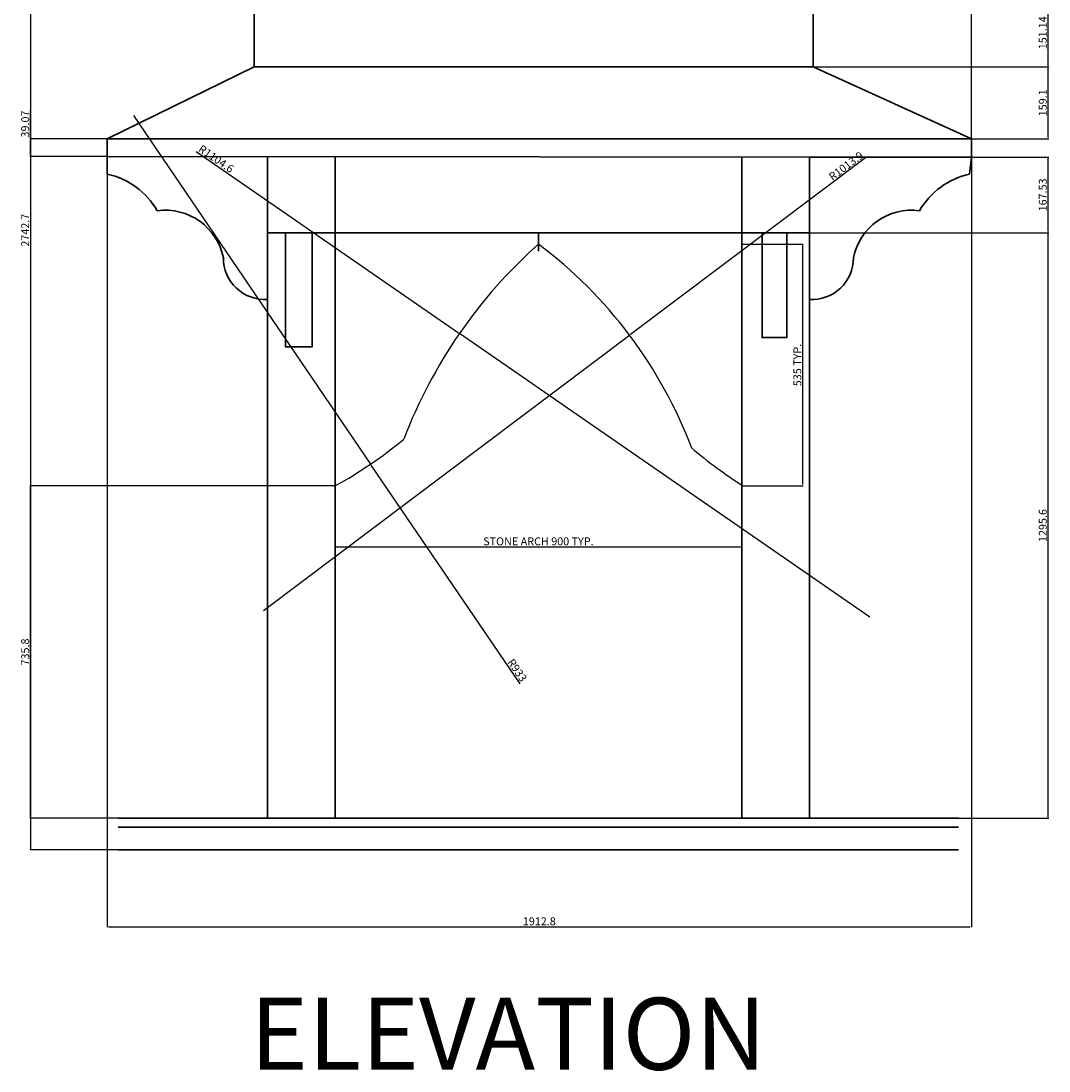
# Model space of a CAD drawing. Units: millimetres. Extents: x 498 to 8860, y -426 to 8717.
# Tile 8 of 9: x 4984 to 7260, y 3757 to 6081. Entities that reach past the tile are written whole.
import ezdxf

# ---------------------------------------------------------------- set-up
doc = ezdxf.new("R2010")
doc.units = ezdxf.units.MM
for name, color, linetype, lineweight in [('A-ANNO-DIMS', 2, 'Continuous', 18), ('A-ANNO-TEXT', 3, 'Continuous', 18), ('A-DETL', 7, 'Continuous', 25), ('A-ELEV', 7, 'Continuous', 35)]:
    doc.layers.add(name, color=color, linetype=linetype, lineweight=lineweight)
doc.styles.get("Standard").update_dxf_attribs({"font": 'arial.ttf'})
doc.dimstyles.new('ISO-25', dxfattribs={"dimtxt": 17.5, "dimasz": 2.5, "dimexe": 1.25, "dimexo": 0.625, "dimtad": 1, "dimdec": 0, "dimtxsty": 'Standard', "dimcen": 2.5, "dimadec": 0, "dimazin": 0, "dimtfac": 1, "dimtdec": 0, "dimtmove": 0, "dimatfit": 3, "dimfxl": 1, "dimarcsym": 0})

# ---------------------------------------------------------------- blocks, each defined once
blk = doc.blocks.new('BRACKET-STONE')
for centre, radius, start, end in [((1183.8, -291.1), 1104.6, 131.6209, 159.0769), ((-158.8, -276), 1013.9, 20.7397, 53.0882), ((-446.2, 819.4), 933, 298.5683, 309.875), ((1523.8, 965), 1147.7, 230.2129, 237.0762)]:
    blk.add_arc(centre, radius, start, end)
blk = doc.blocks.new('*D41')
at = {"layer": 'A-ANNO-DIMS', "color": 0, "lineweight": -2, "transparency": 16777216}
for p, q in [((5679.7, 5051.8), (5679.7, 4916.1)), ((6579.7, 5051.8), (6579.7, 4916.1)), ((5682.2, 4917.4), (6577.2, 4917.4))]:
    blk.add_line(p, q, dxfattribs=at)
at = {"layer": 'A-ANNO-DIMS', "color": 0, "transparency": 16777216}
for points in [[(5682.2, 4917.8), (5682.2, 4917), (5679.7, 4917.4)], [(6577.2, 4917.8), (6577.2, 4917), (6579.7, 4917.4)]]:
    blk.add_solid(points, dxfattribs=at)
at = {"layer": 'Defpoints', "color": 0, "transparency": 16777216}
for p in [(5679.7, 5052.4), (6579.7, 5052.4), (6579.7, 4917.4)]:
    blk.add_point(p, dxfattribs=at)
at = {"layer": 'A-ANNO-DIMS', "color": 0, "transparency": 16777216, "insert": (6129.7, 4927.1), "char_height": 17.5, "attachment_point": 5}
blk.add_mtext('STONE ARCH 900 TYP.', dxfattribs=at)
blk = doc.blocks.new('*D42')
at = {"layer": 'A-ANNO-DIMS', "color": 0, "lineweight": -2, "transparency": 16777216}
for p, q in [((6580.4, 5587.1), (6716, 5587.1)), ((6714.7, 5054.9), (6714.7, 5584.6)), ((6580.4, 5052.4), (6716, 5052.4))]:
    blk.add_line(p, q, dxfattribs=at)
at = {"layer": 'A-ANNO-DIMS', "color": 0, "transparency": 16777216}
for points in [[(6714.3, 5584.6), (6715.1, 5584.6), (6714.7, 5587.1)], [(6714.3, 5054.9), (6715.1, 5054.9), (6714.7, 5052.4)]]:
    blk.add_solid(points, dxfattribs=at)
at = {"layer": 'Defpoints', "color": 0, "transparency": 16777216}
for p in [(6579.7, 5587.1), (6714.7, 5587.1), (6579.7, 5052.4)]:
    blk.add_point(p, dxfattribs=at)
at = {"layer": 'A-ANNO-DIMS', "color": 0, "transparency": 16777216, "insert": (6705.2, 5319.7), "char_height": 17.5, "attachment_point": 5, "rotation": 90}
blk.add_mtext('535 TYP.', dxfattribs=at)
blk = doc.blocks.new('*D52')
at = {"layer": 'A-ANNO-DIMS', "color": 0, "lineweight": -2, "transparency": 16777216}
for p, q in [((5175.3, 5819.6), (5175.3, 4075.4)), ((7088.1, 5819.6), (7088.1, 4075.4)), ((5177.8, 4076.6), (7085.6, 4076.6))]:
    blk.add_line(p, q, dxfattribs=at)
at = {"layer": 'A-ANNO-DIMS', "color": 0, "transparency": 16777216}
for points in [[(5177.8, 4077), (5177.8, 4076.2), (5175.3, 4076.6)], [(7085.6, 4077), (7085.6, 4076.2), (7088.1, 4076.6)]]:
    blk.add_solid(points, dxfattribs=at)
at = {"layer": 'Defpoints', "color": 0, "transparency": 16777216}
for p in [(5175.3, 5820.3), (7088.1, 5820.3), (7088.1, 4076.6)]:
    blk.add_point(p, dxfattribs=at)
at = {"layer": 'A-ANNO-DIMS', "color": 0, "transparency": 16777216, "insert": (6131.7, 4086.2), "char_height": 17.5, "attachment_point": 5}
blk.add_mtext('1912.8', dxfattribs=at)
blk = doc.blocks.new('*D53')
at = {"layer": 'A-ANNO-DIMS', "color": 0, "lineweight": -2, "transparency": 16777216}
for p, q in [((6135.6, 6989.3), (5004.1, 6989.3)), ((5005.3, 6986.8), (5005.3, 4249.1)), ((5199.1, 4246.6), (5004.1, 4246.6))]:
    blk.add_line(p, q, dxfattribs=at)
at = {"layer": 'A-ANNO-DIMS', "color": 0, "transparency": 16777216}
for points in [[(5004.9, 6986.8), (5005.8, 6986.8), (5005.3, 6989.3)], [(5004.9, 4249.1), (5005.8, 4249.1), (5005.3, 4246.6)]]:
    blk.add_solid(points, dxfattribs=at)
at = {"layer": 'Defpoints', "color": 0, "transparency": 16777216}
for p in [(6136.2, 6989.3), (5005.3, 4246.6), (5199.7, 4246.6)]:
    blk.add_point(p, dxfattribs=at)
at = {"layer": 'A-ANNO-DIMS', "color": 0, "transparency": 16777216, "insert": (4995.9, 5617.9), "char_height": 17.5, "attachment_point": 5, "rotation": 90}
blk.add_mtext('2742.7', dxfattribs=at)
blk = doc.blocks.new('*D54')
at = {"layer": 'A-ANNO-DIMS', "color": 0, "lineweight": -2, "transparency": 16777216}
for p, q in [((6730.4, 5612.2), (7259.3, 5612.2)), ((7258.1, 4319.1), (7258.1, 5609.7)), ((6730.4, 4316.6), (7259.3, 4316.6))]:
    blk.add_line(p, q, dxfattribs=at)
at = {"layer": 'A-ANNO-DIMS', "color": 0, "transparency": 16777216}
for points in [[(7257.7, 5609.7), (7258.5, 5609.7), (7258.1, 5612.2)], [(7257.7, 4319.1), (7258.5, 4319.1), (7258.1, 4316.6)]]:
    blk.add_solid(points, dxfattribs=at)
at = {"layer": 'Defpoints', "color": 0, "transparency": 16777216}
for p in [(6729.7, 5612.2), (7258.1, 5612.2), (6729.7, 4316.6)]:
    blk.add_point(p, dxfattribs=at)
at = {"layer": 'A-ANNO-DIMS', "color": 0, "transparency": 16777216, "insert": (7248.5, 4964.4), "char_height": 17.5, "attachment_point": 5, "rotation": 90}
blk.add_mtext('1295.6', dxfattribs=at)
blk = doc.blocks.new('*D55')
at = {"layer": 'A-ANNO-DIMS', "color": 0, "lineweight": -2, "transparency": 16777216}
for p, q in [((6730.4, 5779.7), (7259.3, 5779.7)), ((7258.1, 5614.7), (7258.1, 5777.2)), ((6730.4, 5612.2), (7259.3, 5612.2))]:
    blk.add_line(p, q, dxfattribs=at)
at = {"layer": 'A-ANNO-DIMS', "color": 0, "transparency": 16777216}
for points in [[(7257.7, 5777.2), (7258.5, 5777.2), (7258.1, 5779.7)], [(7257.7, 5614.7), (7258.5, 5614.7), (7258.1, 5612.2)]]:
    blk.add_solid(points, dxfattribs=at)
at = {"layer": 'Defpoints', "color": 0, "transparency": 16777216}
for p in [(6729.7, 5779.7), (7258.1, 5779.7), (6729.7, 5612.2)]:
    blk.add_point(p, dxfattribs=at)
at = {"layer": 'A-ANNO-DIMS', "color": 0, "transparency": 16777216, "insert": (7248.5, 5696), "char_height": 17.5, "attachment_point": 5, "rotation": 90}
blk.add_mtext('167.53', dxfattribs=at)
blk = doc.blocks.new('*D56')
at = {"layer": 'A-ANNO-DIMS', "color": 0, "lineweight": -2, "transparency": 16777216}
for p, q in [((5005.3, 5820.3), (5005.3, 5883.1)), ((5174.7, 5820.3), (5004.1, 5820.3)), ((5005.3, 5783.7), (5005.3, 5817.8)), ((5174.7, 5781.2), (5004.1, 5781.2))]:
    blk.add_line(p, q, dxfattribs=at)
at = {"layer": 'A-ANNO-DIMS', "color": 0, "transparency": 16777216}
for points in [[(5004.9, 5817.8), (5005.8, 5817.8), (5005.3, 5820.3)], [(5004.9, 5783.7), (5005.8, 5783.7), (5005.3, 5781.2)]]:
    blk.add_solid(points, dxfattribs=at)
at = {"layer": 'Defpoints', "color": 0, "transparency": 16777216}
for p in [(5005.3, 5820.3), (5175.3, 5820.3), (5175.3, 5781.2)]:
    blk.add_point(p, dxfattribs=at)
at = {"layer": 'A-ANNO-DIMS', "color": 0, "transparency": 16777216, "insert": (4995.8, 5852.9), "char_height": 17.5, "attachment_point": 5, "rotation": 90}
blk.add_mtext('39.07', dxfattribs=at)
blk = doc.blocks.new('*D57')
at = {"layer": 'A-ANNO-DIMS', "color": 0, "lineweight": -2, "transparency": 16777216}
for p, q in [((6738.5, 5979.4), (7259.3, 5979.4)), ((7258.1, 5822.8), (7258.1, 5976.9)), ((7088.7, 5820.3), (7259.3, 5820.3))]:
    blk.add_line(p, q, dxfattribs=at)
at = {"layer": 'A-ANNO-DIMS', "color": 0, "transparency": 16777216}
for points in [[(7257.7, 5976.9), (7258.5, 5976.9), (7258.1, 5979.4)], [(7257.7, 5822.8), (7258.5, 5822.8), (7258.1, 5820.3)]]:
    blk.add_solid(points, dxfattribs=at)
at = {"layer": 'Defpoints', "color": 0, "transparency": 16777216}
for p in [(6737.8, 5979.4), (7258.1, 5979.4), (7088.1, 5820.3)]:
    blk.add_point(p, dxfattribs=at)
at = {"layer": 'A-ANNO-DIMS', "color": 0, "transparency": 16777216, "insert": (7248.5, 5899.8), "char_height": 17.5, "attachment_point": 5, "rotation": 90}
blk.add_mtext('159.1', dxfattribs=at)
blk = doc.blocks.new('*D58')
at = {"layer": 'A-ANNO-DIMS', "color": 0, "lineweight": -2, "transparency": 16777216}
for p, q in [((6737.8, 5980), (6737.8, 7160.5)), ((6740.3, 7159.3), (7085.6, 7159.3)), ((7088.1, 5820.9), (7088.1, 7160.5))]:
    blk.add_line(p, q, dxfattribs=at)
at = {"layer": 'A-ANNO-DIMS', "color": 0, "transparency": 16777216}
for points in [[(6740.3, 7159.7), (6740.3, 7158.9), (6737.8, 7159.3)], [(7085.6, 7159.7), (7085.6, 7158.9), (7088.1, 7159.3)]]:
    blk.add_solid(points, dxfattribs=at)
at = {"layer": 'Defpoints', "color": 0, "transparency": 16777216}
for p in [(7088.1, 7159.3), (6737.8, 5979.4), (7088.1, 5820.3)]:
    blk.add_point(p, dxfattribs=at)
at = {"layer": 'A-ANNO-DIMS', "color": 0, "transparency": 16777216, "insert": (6913, 7168.8), "char_height": 17.5, "attachment_point": 5}
blk.add_mtext('350.24', dxfattribs=at)
blk = doc.blocks.new('*D59')
at = {"layer": 'A-ANNO-DIMS', "color": 0, "lineweight": -2, "transparency": 16777216}
for p, q in [((6738.5, 6130.5), (7259.3, 6130.5)), ((7258.1, 5981.9), (7258.1, 6128)), ((6738.5, 5979.4), (7259.3, 5979.4))]:
    blk.add_line(p, q, dxfattribs=at)
at = {"layer": 'A-ANNO-DIMS', "color": 0, "transparency": 16777216}
for points in [[(7257.7, 6128), (7258.5, 6128), (7258.1, 6130.5)], [(7257.7, 5981.9), (7258.5, 5981.9), (7258.1, 5979.4)]]:
    blk.add_solid(points, dxfattribs=at)
at = {"layer": 'Defpoints', "color": 0, "transparency": 16777216}
for p in [(6737.8, 6130.5), (7258.1, 6130.5), (6737.8, 5979.4)]:
    blk.add_point(p, dxfattribs=at)
at = {"layer": 'A-ANNO-DIMS', "color": 0, "transparency": 16777216, "insert": (7248.5, 6054.9), "char_height": 17.5, "attachment_point": 5, "rotation": 90}
blk.add_mtext('151.14', dxfattribs=at)
blk = doc.blocks.new('*D63')
at = {"layer": 'A-ANNO-DIMS', "color": 0, "lineweight": -2, "transparency": 16777216}
for p, q in [((5679.1, 5052.4), (5004.1, 5052.4)), ((5005.3, 4319.1), (5005.3, 5049.9)), ((5679.1, 4316.6), (5004.1, 4316.6))]:
    blk.add_line(p, q, dxfattribs=at)
at = {"layer": 'A-ANNO-DIMS', "color": 0, "transparency": 16777216}
for points in [[(5004.9, 5049.9), (5005.8, 5049.9), (5005.3, 5052.4)], [(5004.9, 4319.1), (5005.8, 4319.1), (5005.3, 4316.6)]]:
    blk.add_solid(points, dxfattribs=at)
at = {"layer": 'Defpoints', "color": 0, "transparency": 16777216}
for p in [(5005.3, 5052.4), (5679.7, 5052.4), (5679.7, 4316.6)]:
    blk.add_point(p, dxfattribs=at)
at = {"layer": 'A-ANNO-DIMS', "color": 0, "transparency": 16777216, "insert": (4995.8, 4684.5), "char_height": 17.5, "attachment_point": 5, "rotation": 90}
blk.add_mtext('735.8', dxfattribs=at)
blk = doc.blocks.new('*D81')
at = {"layer": 'A-ANNO-DIMS', "color": 0, "lineweight": -2, "transparency": 16777216}
for p, q in [((5233.5, 5871.8), (5758.3, 5100.3)), ((6089.1, 4614), (5759.7, 5098.3))]:
    blk.add_line(p, q, dxfattribs=at)
at = {"layer": 'A-ANNO-DIMS', "color": 0, "transparency": 16777216}
blk.add_solid([(5760, 5098.5), (5759.3, 5098), (5758.3, 5100.3)], dxfattribs=at)
at = {"layer": 'Defpoints', "color": 0, "transparency": 16777216}
for p in [(5233.5, 5871.8), (5758.3, 5100.3)]:
    blk.add_point(p, dxfattribs=at)
at = {"layer": 'A-ANNO-DIMS', "color": 0, "transparency": 16777216, "insert": (6081, 4642.8), "char_height": 17.5, "attachment_point": 5, "rotation": 304.2213}
blk.add_mtext('R933', dxfattribs=at)
blk = doc.blocks.new('*D82')
at = {"layer": 'A-ANNO-DIMS', "color": 0, "lineweight": -2, "transparency": 16777216}
for p, q in [((6854.1, 5778), (6333.5, 5386.9)), ((5520.9, 4776.4), (6331.5, 5385.4))]:
    blk.add_line(p, q, dxfattribs=at)
at = {"layer": 'A-ANNO-DIMS', "color": 0, "transparency": 16777216}
blk.add_solid([(6333.2, 5387.2), (6333.8, 5386.6), (6331.5, 5385.4)], dxfattribs=at)
at = {"layer": 'Defpoints', "color": 0, "transparency": 16777216}
for p in [(6331.5, 5385.4), (5520.9, 4776.4)]:
    blk.add_point(p, dxfattribs=at)
at = {"layer": 'A-ANNO-DIMS', "color": 0, "transparency": 16777216, "insert": (6812.1, 5758.4), "char_height": 17.5, "attachment_point": 5, "rotation": 36.9171}
blk.add_mtext('R1013.9', dxfattribs=at)
blk = doc.blocks.new('*D83')
at = {"layer": 'A-ANNO-DIMS', "color": 0, "lineweight": -2, "transparency": 16777216}
for p, q in [((5372.3, 5792), (5952.8, 5390.8)), ((6863.5, 4761.3), (5954.8, 5389.4))]:
    blk.add_line(p, q, dxfattribs=at)
at = {"layer": 'A-ANNO-DIMS', "color": 0, "transparency": 16777216}
blk.add_solid([(5953, 5391.1), (5952.5, 5390.5), (5954.8, 5389.4)], dxfattribs=at)
at = {"layer": 'Defpoints', "color": 0, "transparency": 16777216}
for p in [(5954.8, 5389.4), (6863.5, 4761.3)]:
    blk.add_point(p, dxfattribs=at)
at = {"layer": 'A-ANNO-DIMS', "color": 0, "transparency": 16777216, "insert": (5415.1, 5774.1), "char_height": 17.5, "attachment_point": 5, "rotation": 325.3479}
blk.add_mtext('R1104.6', dxfattribs=at)

msp = doc.modelspace()

# ---------------------------------------------------------------- linework, layer by layer
at = {"layer": 'A-ELEV'}
for p, q in [((5175.339, 5820.26), (5500.377, 5979.353)), ((6737.845, 5979.353), (7088.089, 5820.26)), ((5175.339, 5742.114), (5175.339, 5820.26)), ((5175.339, 5820.26), (7088.089, 5820.26)), ((7088.089, 5779.394), (7088.089, 5820.26)), ((5175.339, 5781.187), (7088.089, 5779.394)), ((5529.731, 5612.196), (5529.731, 5780.855)), ((5679.731, 5612.196), (5679.731, 5780.714)), ((6579.731, 5612.196), (6579.731, 5779.871)), ((6729.731, 5612.196), (6729.731, 5779.73)), ((7088.089, 5779.394), (7084.123, 5742.114)), ((5529.731, 4316.61), (5529.731, 5612.196)), ((6129.731, 5612.196), (5529.731, 5612.196)), ((5679.731, 4316.61), (5679.731, 5612.196)), ((6129.731, 5612.196), (6729.731, 5612.196)), ((6129.876, 5571.676), (6129.731, 5612.196)), ((6579.731, 4316.61), (6579.731, 5612.196)), ((6729.731, 4316.61), (6729.731, 5612.196)), ((5199.731, 4316.61), (7059.731, 4316.61)), ((5199.731, 4296.61), (7059.731, 4296.61)), ((5199.731, 4246.61), (7059.731, 4246.61))]:
    msp.add_line(p, q, dxfattribs=at)
for points in [[(5500.377, 6130.498), (6737.845, 6130.498), (6737.845, 5979.353), (5500.377, 5979.353)], [(5570.062, 5612.196), (5628.657, 5612.196), (5628.657, 5359.74), (5570.062, 5359.74)], [(6624.905, 5612.196), (6679.463, 5612.196), (6679.463, 5380.346), (6624.905, 5380.346)]]:
    msp.add_lwpolyline(points, close=True, dxfattribs=at)
for centre, radius, start, end in [((5137.323, 5574.109), 172.253, 30.289705, 77.249938), ((7122.139, 5574.109), 172.253, 102.750062, 149.710295), ((5303.725, 5531.128), 131.056, 11.188127, 97.745996), ((6955.736, 5531.128), 131.056, 82.254004, 168.811873), ((5524.231, 5556.557), 91.941, 180, 273.429009), ((6735.23, 5556.557), 91.941, 266.570991, 0)]:
    msp.add_arc(centre, radius, start, end, dxfattribs=at)

# ---------------------------------------------------------------- block references
at = {"layer": 'A-DETL'}
msp.add_blockref('BRACKET-STONE', (5679.731, 5052.395), dxfattribs=at)

# ---------------------------------------------------------------- texts
at = {"layer": 'A-ANNO-TEXT'}
msp.add_text('ELEVATION', height=159.2, dxfattribs=at).set_placement((5491.731, 3760.055))

# ---------------------------------------------------------------- dimensions: what is measured, and where the dimension line sits
at = {"layer": 'A-ANNO-DIMS'}
for base, p1, p2, override, picture, middle in [((7088.089, 7159.279), (6737.845, 5979.353), (7088.089, 5820.26), {"dimdec": 2, "dimlfac": 1, "dimrnd": 0, "dimzin": 0, "dimdsep": 46, "dimlunit": 2}, '*D58', (6912.967, 7168.845)), ((7088.0889, 4076.61), (5175.3386, 5820.26), (7088.0889, 5820.26), {"dimdec": 1, "dimlfac": 1, "dimrnd": 0, "dimzin": 0, "dimdsep": 46, "dimlunit": 2}, '*D52', (6131.7138, 4086.17))]:
    dim = msp.add_linear_dim(base=base, p1=p1, p2=p2, dimstyle='ISO-25', override=override, dxfattribs=at)
    dim.commit()
    dim.dimension.update_dxf_attribs({"geometry": picture, "text_midpoint": middle})
for base, p1, p2, override, picture, middle in [((5005.339, 4246.61), (6136.19, 6989.279), (5199.731, 4246.61), {"dimdec": 1, "dimlfac": 1, "dimrnd": 0, "dimzin": 0, "dimdsep": 46, "dimlunit": 2}, '*D53', (4995.928, 5617.944)), ((7258.0889, 6130.49787), (6737.84498, 5979.35295), (6737.84498, 6130.49787), {"dimdec": 2, "dimlfac": 1, "dimrnd": 0, "dimzin": 0, "dimdsep": 46, "dimlunit": 2}, '*D59', (7248.52888, 6054.92541)), ((7258.089, 5979.353), (7088.089, 5820.26), (6737.845, 5979.353), {"dimdec": 1, "dimlfac": 1, "dimrnd": 0, "dimzin": 0, "dimdsep": 46, "dimlunit": 2}, '*D57', (7248.529, 5899.806)), ((5005.339, 5820.26), (5175.339, 5781.187), (5175.339, 5820.26), {"dimdec": 2, "dimlfac": 1, "dimrnd": 0, "dimzin": 0, "dimdsep": 46, "dimlunit": 2}, '*D56', (4995.773, 5852.906)), ((7258.089, 5779.73), (6729.731, 5612.196), (6729.731, 5779.73), {"dimdec": 2, "dimlfac": 1, "dimrnd": 0, "dimzin": 0, "dimdsep": 46, "dimlunit": 2}, '*D55', (7248.523, 5695.963)), ((7258.089, 5612.196), (6729.731, 4316.61), (6729.731, 5612.196), {"dimdec": 1, "dimlfac": 1, "dimrnd": 0, "dimzin": 0, "dimdsep": 46, "dimlunit": 2}, '*D54', (7248.529, 4964.403)), ((5005.339, 5052.396), (5679.731, 4316.61), (5679.731, 5052.396), {"dimdec": 1, "dimlfac": 1, "dimrnd": 0, "dimzin": 0, "dimdsep": 46, "dimlunit": 2}, '*D63', (4995.773, 4684.503))]:
    dim = msp.add_linear_dim(base=base, p1=p1, p2=p2, angle=90, dimstyle='ISO-25', override=override, dxfattribs=at)
    dim.commit()
    dim.dimension.update_dxf_attribs({"geometry": picture, "text_midpoint": middle})
for center, mpoint, override, picture, middle in [((5233.548, 5871.832), (5758.278, 5100.332), {"dimdec": 0, "dimlfac": 1, "dimrnd": 0, "dimzin": 0, "dimdsep": 46, "dimlunit": 2}, '*D81', (6073.117, 4637.432)), ((6863.5, 4761.309), (5954.83, 5389.379), {"dimdec": 1, "dimlfac": 1, "dimrnd": 0, "dimzin": 0, "dimdsep": 46, "dimlunit": 2}, '*D83', (5409.628, 5766.222)), ((5520.905, 4776.409), (6331.502, 5385.401), {"dimdec": 1, "dimlfac": 1, "dimrnd": 0, "dimzin": 0, "dimdsep": 46, "dimlunit": 2}, '*D82', (6817.86, 5750.796))]:
    dim = msp.add_radius_dim(center=center, mpoint=mpoint, dimstyle='ISO-25', override=override, dxfattribs=at)
    dim.commit()
    dim.dimension.update_dxf_attribs({"geometry": picture, "text_midpoint": middle, "dimtype": 164})
dim = msp.add_linear_dim(base=(6714.731, 5587.063), p1=(6579.731, 5052.396), p2=(6579.731, 5587.063), angle=90, text='<> TYP.', dimstyle='ISO-25', override={"dimdec": 0, "dimrnd": 0, "dimzin": 0, "dimlunit": 2}, dxfattribs=at)
dim.commit()
dim.dimension.update_dxf_attribs({"geometry": '*D42', "text_midpoint": (6705.165, 5319.729)})
dim = msp.add_linear_dim(base=(6579.731, 4917.396), p1=(5679.731, 5052.396), p2=(6579.731, 5052.396), text='STONE ARCH <> TYP.', dimstyle='ISO-25', override={"dimdec": 0, "dimrnd": 0, "dimzin": 0, "dimlunit": 2}, dxfattribs=at)
dim.commit()
dim.dimension.update_dxf_attribs({"geometry": '*D41', "text_midpoint": (6129.731, 4927.075)})

doc.saveas('drawing.dxf')
